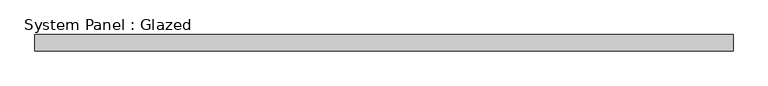
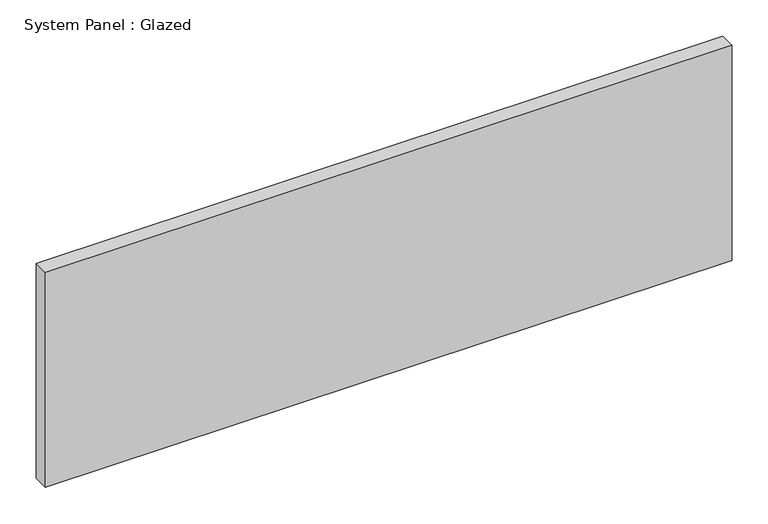
"""IFC4 building model written with IfcOpenShell, lengths in millimetres: plate geometry, System Panel : Glazed."""

from ifc_helpers import new_model, si_unit, origin, origin_with_axes, place, context, project, spatial, polyline, outline, extrude, source, transform, mapped, element, save


def system_panel_glazed_a38391a9(model_context):
    return source(origin(), model_context, "Body", "SweptSolid", [
        extrude(outline(polyline([(546.1, 19.05), (-546.1, 19.05), (-546.1, 44.45), (546.1, 44.45), (546.1, 19.05)])), origin_with_axes(), (0.0, 0.0, 1.0), 361.95),
    ])


if __name__ == "__main__":
    model = new_model("IFC4")
    model_context = context("Model", 3, world=origin())
    ifc_project = project(units=[si_unit("LENGTHUNIT", "METRE", prefix="MILLI")], contexts=[model_context])
    site = spatial("IfcSite", under=ifc_project)
    building = spatial("IfcBuilding", under=site)
    placement = place(None, origin())
    system_panel_glazed_shape = system_panel_glazed_a38391a9(model_context)
    element("IfcPlate", 1, ObjectType="System Panel : Glazed", at=placement, inside=building, context=model_context, shape_type="MappedRepresentation", body=[
        mapped(system_panel_glazed_shape, transform((0.0, 0.0, 0.0), x_axis=(1.0, 0.0, 0.0), y_axis=(0.0, 1.0, 0.0), z_axis=(0.0, 0.0, 1.0))),
    ])
    save(model, "model.ifc")

# Revit data of these elements
# Type "System Panel : Glazed"
#   Construction Type Id = "GSP4R"
#   Analytic Construction = "1/8 in Pilkington single glazing"
#   Visual Light Transmittance = 0.9
#   Solar Heat Gain Coefficient = 0.86
#   Heat Transfer Coefficient (U) = 1.18115 BTU/(h·ft²·°F)
#   Define Thermal Properties by = 1
# Element 1 (IfcPlate, "System Panel : Glazed")
#   Materials on its faces: "Glass"
# Materials
#   "Glass": class "Glass", colour RGB 0 128 192, transparency 0.75, Description = "Soda Lime Glass", Cost = 0
